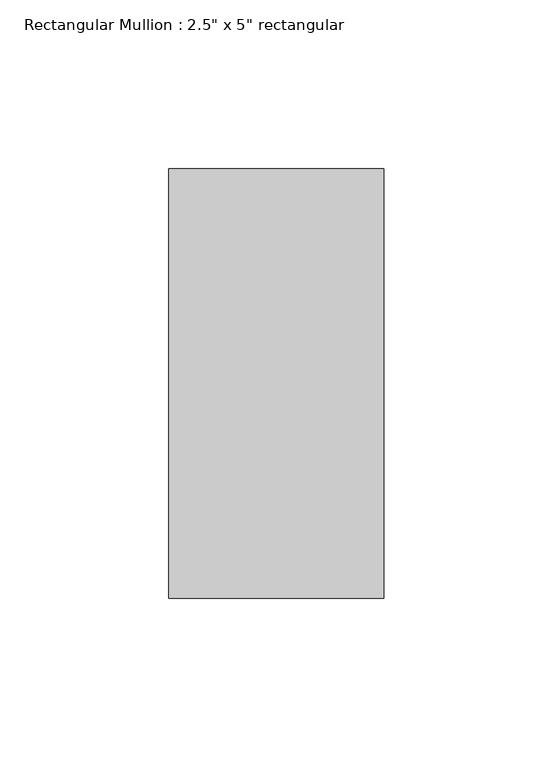
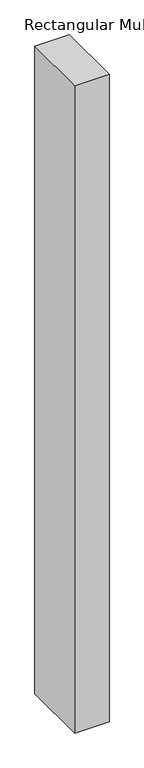
"""IFC4 building model written with IfcOpenShell, lengths in millimetres: member geometry."""

from ifc_helpers import new_model, si_unit, frame, origin, place, context, project, spatial, polyline, outline, extrude, source, transform, mapped, element, save


def member_0d684f40(model_context):
    return source(origin(), model_context, "Body", "SweptSolid", [
        extrude(outline(polyline([(0.0, 63.5), (0.0, -63.5), (-63.5, -63.5), (-63.5, 63.5), (0.0, 63.5)])), frame((0.0, 0.0, -1262.7052325), z_axis=(0.0, 0.0, 1.0), x_axis=(1.0, 0.0, 0.0)), (0.0, 0.0, 1.0), 1262.7052325),
    ])


if __name__ == "__main__":
    model = new_model("IFC4")
    model_context = context("Model", 3, world=origin())
    ifc_project = project(units=[si_unit("LENGTHUNIT", "METRE", prefix="MILLI")], contexts=[model_context])
    site = spatial("IfcSite", under=ifc_project)
    building = spatial("IfcBuilding", under=site)
    placement = place(None, origin())
    member_shape = member_0d684f40(model_context)
    element("IfcMember", 1, ObjectType="Rectangular Mullion : 2.5\" x 5\" rectangular", at=placement, inside=building, context=model_context, shape_type="MappedRepresentation", body=[
        mapped(member_shape, transform((0.0, 0.0, 0.0), x_axis=(1.0, 0.0, 0.0), y_axis=(0.0, 1.0, 0.0), z_axis=(0.0, 0.0, 1.0))),
    ])
    save(model, "model.ifc")

# Revit data of these elements
# Type "Rectangular Mullion : 2.5\" x 5\" rectangular"
#   built-in parameter 1007304 = 0.416667 (stored number, unit not read)
#   built-in parameter 1007301 = 0.104167 (stored number, unit not read)
#   built-in parameter 1007300 = 0.104167 (stored number, unit not read)
# Element 1 (IfcMember, "Rectangular Mullion : 2.5\" x 5\" rectangular")
#   Materials on its faces: "Iron, Ductile"
# Materials
#   "Iron, Ductile": class "Metal", colour RGB 0 0 0, transparency 0, Description = "Ductile cast iron", Cost = 0
